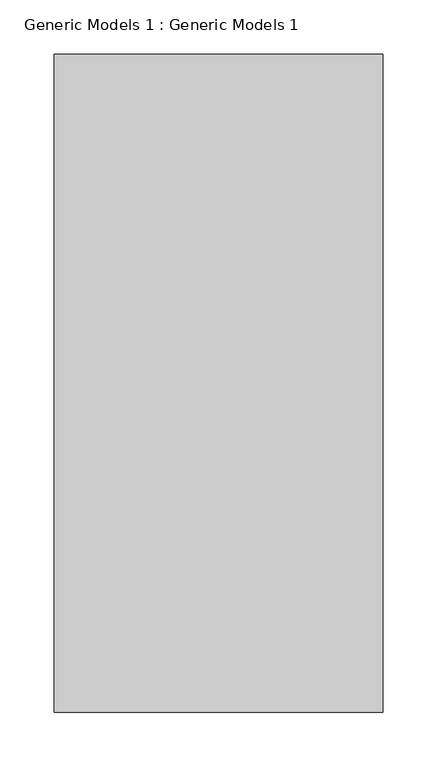
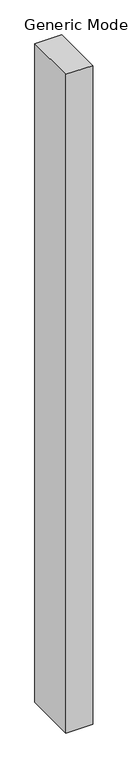
"""IFC4 building model written with IfcOpenShell, lengths in millimetres: proxy geometry, Generic Models 1 : Generic Models 1."""

from ifc_helpers import new_model, si_unit, origin, origin_with_axes, place, context, project, spatial, polyline, outline, extrude, source, transform, mapped, element, save


def generic_models_1_generic_models_1_d450fbd8(model_context):
    return source(origin(), model_context, "Body", "SweptSolid", [
        extrude(outline(polyline([(-8452.845593, -4721.074389), (-8757.645593, -4721.074389), (-8757.645593, -4111.474389), (-8452.845593, -4111.474389), (-8452.845593, -4721.074389)])), origin_with_axes(), (0.0, 0.0, 1.0), 7924.8),
    ])


if __name__ == "__main__":
    model = new_model("IFC4")
    model_context = context("Model", 3, world=origin())
    ifc_project = project(units=[si_unit("LENGTHUNIT", "METRE", prefix="MILLI")], contexts=[model_context])
    site = spatial("IfcSite", under=ifc_project)
    building = spatial("IfcBuilding", under=site)
    placement = place(None, origin())
    generic_models_1_generic_models_1_shape = generic_models_1_generic_models_1_d450fbd8(model_context)
    element("IfcBuildingElementProxy", 1, Name="Generic Models 1 : Generic Models 1", ObjectType="Generic Models 1 : Generic Models 1", at=placement, inside=building, context=model_context, shape_type="MappedRepresentation", body=[
        mapped(generic_models_1_generic_models_1_shape, transform((0.0, 0.0, 0.0), x_axis=(1.0, 0.0, 0.0), y_axis=(0.0, 1.0, 0.0), z_axis=(0.0, 0.0, 1.0))),
    ])
    save(model, "model.ifc")
